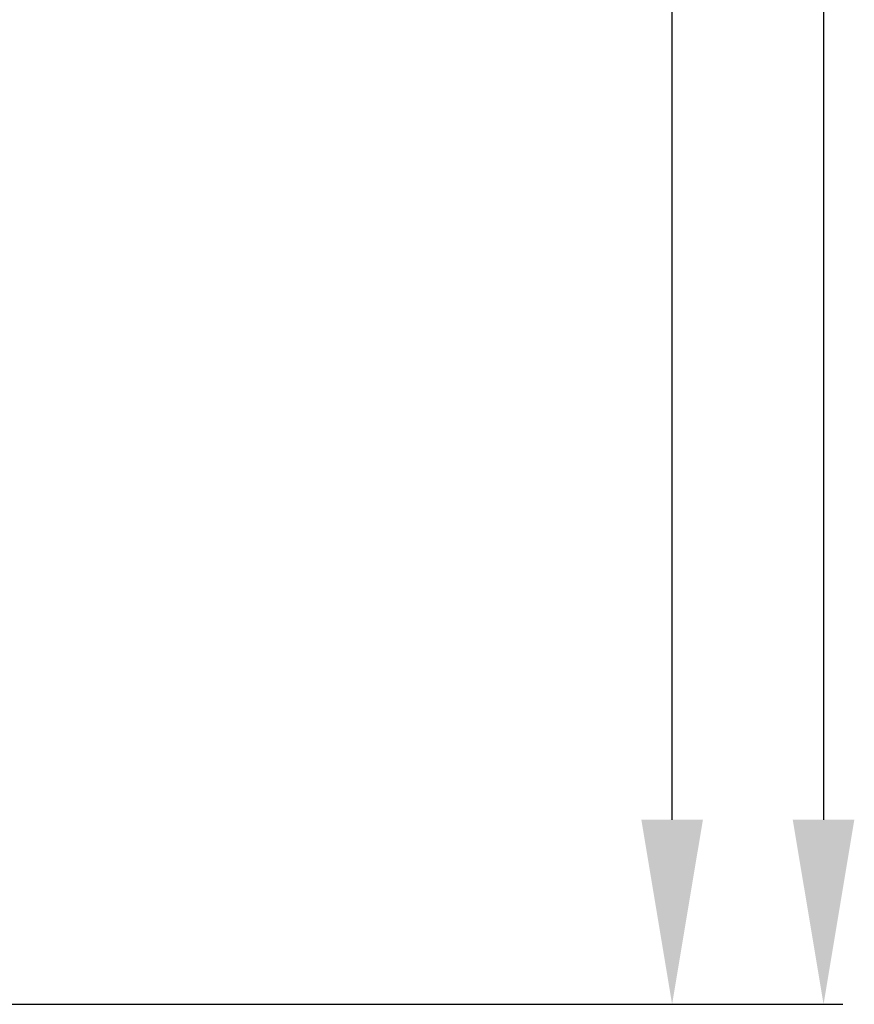
# Model space of a CAD drawing. Units: inches. Extents: x 2083 to 3317, y 1141 to 2115.
# Tile 241 of 256: x 3137 to 3191, y 1263 to 1327. Entities that reach past the tile are written whole.
import ezdxf

# ---------------------------------------------------------------- set-up
doc = ezdxf.new("R2010")
doc.units = ezdxf.units.IN
doc.layers.add('A-ANNO-DIMS', color=2, linetype='Continuous', lineweight=18)
doc.styles.get("Standard").update_dxf_attribs({"font": 'arial.ttf'})
doc.dimstyles.new('ISO-25', dxfattribs={"dimtxt": 12, "dimasz": 12, "dimexe": 1.25, "dimexo": 0.625, "dimtad": 1, "dimlunit": 3, "dimtxsty": 'Standard', "dimcen": 2.5, "dimadec": 0, "dimazin": 0, "dimtfac": 1, "dimtmove": 0, "dimatfit": 3, "dimfxl": 1, "dimarcsym": 0})

# ---------------------------------------------------------------- blocks, each defined once
blk = doc.blocks.new('*D9')
at = {"layer": 'A-ANNO-DIMS', "color": 0, "lineweight": -2, "transparency": 16777216}
for p, q in [((3127.585, 1486.761), (3190.403, 1486.761)), ((3189.153, 1474.761), (3189.153, 1275.261)), ((3127.585, 1263.261), (3190.403, 1263.261))]:
    blk.add_line(p, q, dxfattribs=at)
at = {"layer": 'A-ANNO-DIMS', "color": 0, "transparency": 16777216}
for points in [[(3187.153, 1474.761), (3191.153, 1474.761), (3189.153, 1486.761)], [(3187.153, 1275.261), (3191.153, 1275.261), (3189.153, 1263.261)]]:
    blk.add_solid(points, dxfattribs=at)
at = {"layer": 'Defpoints', "color": 0, "transparency": 16777216}
for p in [(3126.96, 1486.761), (3126.96, 1263.261), (3189.153, 1263.261)]:
    blk.add_point(p, dxfattribs=at)
at = {"layer": 'A-ANNO-DIMS', "color": 0, "transparency": 16777216, "insert": (3182.401, 1375.011), "char_height": 12, "attachment_point": 5, "rotation": 90}
blk.add_mtext('18\'-7.5"', dxfattribs=at)
blk = doc.blocks.new('*D35')
at = {"layer": 'A-ANNO-DIMS', "color": 0, "lineweight": -2, "transparency": 16777216}
for p, q in [((3127.585, 2020.761), (3180.56, 2020.761)), ((3179.31, 1275.261), (3179.31, 2008.761)), ((3127.585, 1263.261), (3180.56, 1263.261))]:
    blk.add_line(p, q, dxfattribs=at)
at = {"layer": 'A-ANNO-DIMS', "color": 0, "transparency": 16777216}
for points in [[(3177.31, 2008.761), (3181.31, 2008.761), (3179.31, 2020.761)], [(3177.31, 1275.261), (3181.31, 1275.261), (3179.31, 1263.261)]]:
    blk.add_solid(points, dxfattribs=at)
at = {"layer": 'Defpoints', "color": 0, "transparency": 16777216}
for p in [(3126.96, 2020.761), (3179.31, 2020.761), (3126.96, 1263.261)]:
    blk.add_point(p, dxfattribs=at)
at = {"layer": 'A-ANNO-DIMS', "color": 0, "transparency": 16777216, "insert": (3172.476, 1642.011), "char_height": 12, "attachment_point": 5, "rotation": 90}
blk.add_mtext('63\'-1 1/2"', dxfattribs=at)

msp = doc.modelspace()

# ---------------------------------------------------------------- dimensions: what is measured, and where the dimension line sits
at = {"layer": 'A-ANNO-DIMS'}
for base, p1, p2, override, picture, middle in [((3179.31, 2020.761), (3126.96, 1263.261), (3126.96, 2020.761), {"dimdec": 1, "dimlfac": 1, "dimrnd": 0, "dimzin": 1, "dimdsep": 46, "dimlunit": 4, "dimfrac": 2}, '*D35', (3172.476, 1642.011)), ((3189.153, 1263.261), (3126.96, 1486.761), (3126.96, 1263.261), {"dimclrd": 0, "dimclre": 0, "dimclrt": 0}, '*D9', (3182.401, 1375.011))]:
    dim = msp.add_linear_dim(base=base, p1=p1, p2=p2, angle=90, dimstyle='ISO-25', override=override, dxfattribs=at)
    dim.commit()
    dim.dimension.update_dxf_attribs({"geometry": picture, "text_midpoint": middle})

doc.saveas('drawing.dxf')
